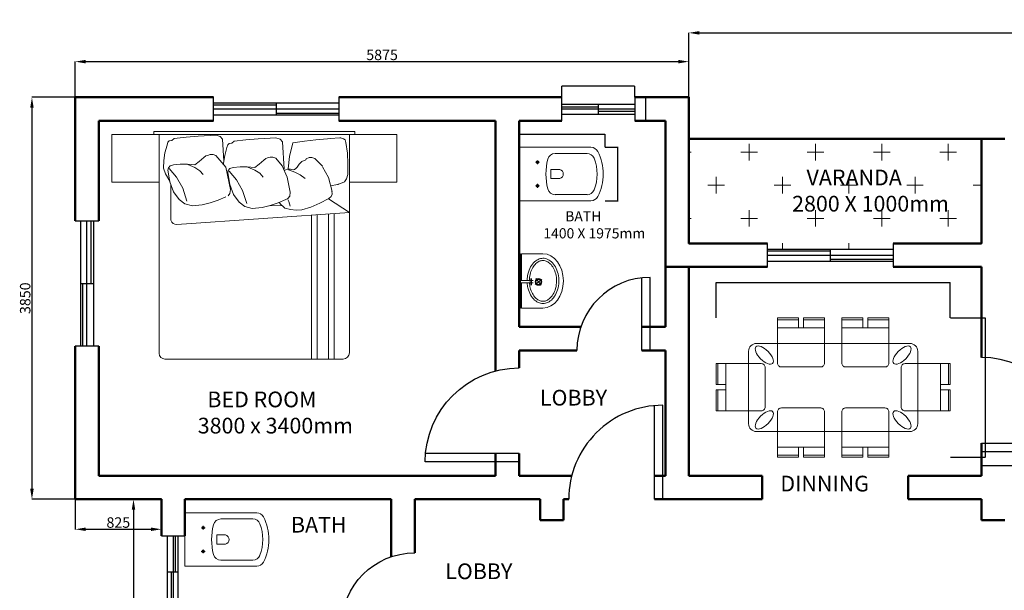
# Model space of a CAD drawing. Units: millimetres. Extents: x -857 to 54106, y -13666 to 13947.
# Tile 11 of 41: x 2211 to 11637, y 8482 to 13947. Entities that reach past the tile are written whole.
import ezdxf

# ---------------------------------------------------------------- set-up
doc = ezdxf.new("R2010")
doc.units = ezdxf.units.MM
for name, color, linetype, lineweight in [('A-ANNO-DIMS', 2, 'Continuous', 18), ('A-AREA-IDEN', 3, 'Continuous', 18), ('A-DOOR', 1, 'Continuous', 25), ('A-FLOR-FIXT', 8, 'Continuous', 18), ('A-FLOR-PATT', 252, 'Continuous', 13), ('A-FURN', 21, 'Continuous', 18), ('A-FURNITURE', 25, 'Continuous', 9), ('A-GLAZ', 4, 'Continuous', 25), ('A-SANITARY FITTINGS', 25, 'Continuous', 15), ('A-WALL', 7, 'Continuous', 50)]:
    doc.layers.add(name, color=color, linetype=linetype, lineweight=lineweight)
doc.styles.get("Standard").update_dxf_attribs({"font": 'arial.ttf'})
doc.dimstyles.new('ISO-25', dxfattribs={"dimtxt": 2.5, "dimasz": 2.5, "dimexe": 1.25, "dimexo": 0.625, "dimtad": 1, "dimtxsty": 'Standard', "dimcen": 2.5, "dimadec": 0, "dimazin": 0, "dimtfac": 1, "dimtmove": 0, "dimatfit": 3, "dimfxl": 1, "dimarcsym": 0})

# ---------------------------------------------------------------- blocks, each defined once
blk = doc.blocks.new('dasd')
at = {"layer": 'A-FURNITURE'}
for p, q in [((-12.51, 13.31), (-12.51, 2.88)), ((-3.95, 13.31), (-12.51, 13.31)), ((-3.95, 12.51), (-12.51, 12.51)), ((-3.95, 9.3), (-3.95, 13.31)), ((6.74, 13.31), (-1.81, 13.31)), ((-1.81, 9.3), (-1.81, 13.31)), ((6.74, 12.51), (-1.81, 12.51)), ((6.74, 2.88), (6.74, 13.31)), ((6.74, 9.3), (-12.51, 9.3)), ((-21, -11.75), (-31.43, -11.75)), ((-31.43, -11.75), (-31.43, -20.3)), ((-30.63, -11.75), (-30.63, -20.3)), ((-27.42, -11.75), (-27.42, -31)), ((15, -11.75), (25.43, -11.75)), ((21.42, -11.75), (21.42, -31)), ((24.63, -11.75), (24.63, -20.3)), ((25.43, -11.75), (25.43, -20.3)), ((-27.42, -20.3), (-31.43, -20.3)), ((-31.43, -22.44), (-31.43, -31)), ((-27.42, -22.44), (-31.43, -22.44)), ((-30.63, -22.44), (-30.63, -31)), ((21.42, -20.3), (25.43, -20.3)), ((21.42, -22.44), (25.43, -22.44)), ((24.63, -22.44), (24.63, -31)), ((25.43, -22.44), (25.43, -31)), ((-31.43, -31), (-21, -31)), ((25.43, -31), (15, -31)), ((-21, -38), (-31.43, -38)), ((-31.43, -38), (-31.43, -46.55)), ((-30.63, -38), (-30.63, -46.55)), ((-27.42, -38), (-27.42, -57.25)), ((15, -38), (25.43, -38)), ((21.42, -38), (21.42, -57.25)), ((24.63, -38), (24.63, -46.55)), ((25.43, -38), (25.43, -46.55)), ((-27.42, -46.55), (-31.43, -46.55)), ((21.42, -46.55), (25.43, -46.55)), ((-31.43, -48.69), (-31.43, -57.25)), ((-27.42, -48.69), (-31.43, -48.69)), ((-30.63, -48.69), (-30.63, -57.25)), ((21.42, -48.69), (25.43, -48.69)), ((24.63, -48.69), (24.63, -57.25)), ((25.43, -48.69), (25.43, -57.25)), ((-31.43, -57.25), (-21, -57.25)), ((25.43, -57.25), (15, -57.25)), ((-12.51, -82.31), (-12.51, -71.88)), ((6.74, -71.88), (6.74, -82.31)), ((6.74, -78.3), (-12.51, -78.3)), ((-3.95, -78.3), (-3.95, -82.31)), ((-1.81, -78.3), (-1.81, -82.31)), ((-3.95, -81.51), (-12.51, -81.51)), ((-3.95, -82.31), (-12.51, -82.31)), ((6.74, -81.51), (-1.81, -81.51)), ((6.74, -82.31), (-1.81, -82.31))]:
    blk.add_line(p, q, dxfattribs=at)
blk.add_lwpolyline([(-21, -65.79), (-21, -3.21, -0.414214), (-17.79, 0), (11.79, 0, -0.414214), (15, -3.21), (15, -65.79, -0.414214), (11.79, -69), (-17.79, -69, -0.414214)], format="xyb", close=True, dxfattribs=at)
at = {"layer": 'A-FURNITURE', "ltscale": 5}
for points in [[(-12.51, 2.88), (-12.51, -5.14, 0.414214), (-10.91, -6.74), (5.14, -6.74, 0.414214), (6.74, -5.14), (6.74, 2.88)], [(-21, -31), (-12.98, -31, 0.414214), (-11.37, -29.4), (-11.37, -13.35, 0.414214), (-12.98, -11.75), (-21, -11.75)], [(15, -31), (6.98, -31, -0.414214), (5.37, -29.4), (5.37, -13.35, -0.414214), (6.98, -11.75), (15, -11.75)], [(-21, -57.25), (-12.98, -57.25, 0.414214), (-11.37, -55.65), (-11.37, -39.6, 0.414214), (-12.98, -38), (-21, -38)], [(15, -57.25), (6.98, -57.25, -0.414214), (5.37, -55.65), (5.37, -39.6, -0.414214), (6.98, -38), (15, -38)], [(-12.51, -71.88), (-12.51, -63.86, -0.414214), (-10.91, -62.26), (5.14, -62.26, -0.414214), (6.74, -63.86), (6.74, -71.88)]]:
    blk.add_lwpolyline(points, format="xyb", dxfattribs=at)
for centre, major_axis in [((-16.23, -6.4), (-3.4, 3.4)), ((10.23, -62.6), (3.4, -3.4))]:
    blk.add_ellipse(centre, major_axis=major_axis, ratio=0.444444, dxfattribs=at)
at = {"layer": 'A-FURNITURE', "ltscale": 5, "extrusion": (0, 0, -1)}
for centre, major_axis in [((10.23, -6.4), (3.4, 3.4)), ((-16.23, -62.6), (-3.4, -3.4))]:
    blk.add_ellipse(centre, major_axis=major_axis, ratio=0.444444, dxfattribs=at)
blk = doc.blocks.new('A$C7d9d00ca')
at = {"layer": 'A-SANITARY FITTINGS'}
for p, q in [((0, 0), (-13.78, 0)), ((-13.78, -18.49), (-13.78, 0)), ((0, -18.49), (0, 0)), ((-10.42, -4.72), (-9.43, -4.72)), ((-9.94, -4.23), (-9.94, -5.23)), ((-3.36, -4.73), (-4.34, -4.73)), ((-3.84, -4.24), (-3.84, -5.24)), ((-12.2, -9.27), (-12.2, -17.48)), ((-1.57, -9.27), (-1.57, -17.48))]:
    blk.add_line(p, q, dxfattribs=at)
for points in [[(-8.08, -8.19), (-5.7, -8.19), (-5.7, -8.19), (-5.7, -10.48)], [(-8.08, -8.19), (-8.08, -10.48)]]:
    blk.add_lwpolyline(points, dxfattribs=at)
for centre in [(-9.94, -4.72), (-3.84, -4.73)]:
    blk.add_circle(centre, 0.342, dxfattribs=at)
for centre, radius, start, end in [((-10.24, -9.27), 1.97, 103.8652, 180), ((-6.89, -22.82), 15.93, 76.135, 103.8652), ((-3.54, -9.27), 1.97, 0.0003, 76.135), ((-6.89, -10.13), 1.24, 196.5098, 343.4902), ((-10.24, -17.48), 1.97, 180, 248.6555), ((-3.54, -17.48), 1.97, 291.3447, 0.0003), ((-11.81, -18.49), 1.97, 180, 242.8074), ((-6.89, -8.92), 12.74, 242.8074, 297.1926), ((-6.89, -8.92), 11.16, 248.6555, 291.3447), ((-1.97, -18.49), 1.97, 297.1926, 0)]:
    blk.add_arc(centre, radius, start, end, dxfattribs=at)
blk = doc.blocks.new('A$C0124305E')
at = {"layer": 'A-SANITARY FITTINGS'}
for p, q in [((-8.42, 16.01), (-0.8, 16.01)), ((-0.8, 7.08), (-0.8, 16.01)), ((-5.66, 7.68), (-8, 5.88)), ((-7.73, 7.95), (-5.93, 5.62)), ((0, 7.08), (-4.99, 7.08)), ((-4.31, 5.61), (-4.31, 7.96)), ((-3.91, 5.61), (-3.91, 7.96)), ((0, 6.28), (-4.99, 6.28)), ((-0.8, -3.19), (-0.8, 6.28)), ((-8.42, -3.19), (-0.8, -3.19))]:
    blk.add_line(p, q, dxfattribs=at)
blk.add_lwpolyline([(-0.5, 16.01), (0, 16.01), (0, -3.19), (-0.5, -3.19)], close=True, dxfattribs=at)
for radius in [1.18, 0.885]:
    blk.add_circle((-6.83, 6.78), radius, dxfattribs=at)
at = {"layer": 'A-SANITARY FITTINGS', "extrusion": (0, 0, -1)}
blk.add_ellipse((-8.42, 6.41), major_axis=(0, 9.6), ratio=0.75, start_param=3.141593, end_param=6.283185, dxfattribs=at)
at = {"layer": 'A-SANITARY FITTINGS'}
for points, knots in [([(-2.82, 6.28), (-2.82, 5.74), (-2.87, 5.2), (-3.1, 3.74), (-3.37, 2.86), (-4.09, 1.28), (-4.55, 0.6), (-5.56, -0.5), (-6.12, -0.92), (-7.25, -1.45), (-7.83, -1.58), (-8.98, -1.59), (-9.55, -1.46), (-10.69, -0.93), (-11.25, -0.52), (-12.27, 0.57), (-12.72, 1.25), (-13.45, 2.82), (-13.72, 3.71), (-14.02, 5.56), (-14.05, 6.52), (-13.88, 8.41), (-13.67, 9.32), (-13.04, 10.99), (-12.62, 11.73), (-11.66, 12.96), (-11.12, 13.45), (-10, 14.13), (-9.43, 14.32), (-8.28, 14.45), (-7.7, 14.39), (-6.56, 14), (-5.99, 13.66), (-4.93, 12.71), (-4.44, 12.09), (-3.62, 10.62), (-3.3, 9.78), (-2.96, 8.29), (-2.87, 7.69), (-2.84, 7.08)], [1.58652, 1.58652, 1.58652, 1.58652, 1.780321, 1.780321, 2.120053, 2.120053, 2.459785, 2.459785, 2.799517, 2.799517, 3.139249, 3.139249, 3.478981, 3.478981, 3.818713, 3.818713, 4.158445, 4.158445, 4.498177, 4.498177, 4.837909, 4.837909, 5.177641, 5.177641, 5.517373, 5.517373, 5.857105, 5.857105, 6.196837, 6.196837, 6.536569, 6.536569, 6.876301, 6.876301, 7.216033, 7.216033, 7.555765, 7.555765, 7.774364, 7.774364, 7.774364, 7.774364]), ([(-3.62, 6.29), (-3.62, 5.76), (-3.67, 5.23), (-3.88, 3.96), (-4.1, 3.23), (-4.65, 1.95), (-4.98, 1.39), (-5.72, 0.46), (-6.12, 0.1), (-6.92, -0.44), (-7.32, -0.61), (-8.11, -0.8), (-8.5, -0.81), (-9.28, -0.69), (-9.68, -0.55), (-10.48, -0.08), (-10.89, 0.24), (-11.67, 1.13), (-12.05, 1.7), (-12.66, 3.01), (-12.9, 3.76), (-13.2, 5.38), (-13.25, 6.28), (-13.13, 8.02), (-12.95, 8.88), (-12.42, 10.42), (-12.06, 11.12), (-11.23, 12.25), (-10.77, 12.7), (-9.92, 13.26), (-9.53, 13.43), (-8.78, 13.62), (-8.41, 13.64), (-7.66, 13.54), (-7.28, 13.42), (-6.51, 13.02), (-6.12, 12.73), (-5.35, 11.95), (-4.97, 11.43), (-4.34, 10.23), (-4.08, 9.54), (-3.76, 8.24), (-3.67, 7.64), (-3.63, 7.03)], [1.58652, 1.58652, 1.58652, 1.58652, 1.790653, 1.790653, 2.093007, 2.093007, 2.384527, 2.384527, 2.676047, 2.676047, 2.967567, 2.967567, 3.259087, 3.259087, 3.550608, 3.550608, 3.842128, 3.842128, 4.155456, 4.155456, 4.468784, 4.468784, 4.806699, 4.806699, 5.144614, 5.144614, 5.482529, 5.482529, 5.820444, 5.820444, 6.099515, 6.099515, 6.378586, 6.378586, 6.657656, 6.657656, 6.936727, 6.936727, 7.23864, 7.23864, 7.540552, 7.540552, 7.774364, 7.774364, 7.774364, 7.774364])]:
    blk.add_open_spline(points, degree=3, knots=knots, dxfattribs=at)
blk = doc.blocks.new('A$C06e6df2d')
at = {"layer": 'A-FURNITURE'}
for p, q in [((-75.01, 24.58), (-75.01, 68.89)), ((-73.01, 70.89), (-16.87, 70.89)), ((-70.22, 24.92), (-70.22, 70.89)), ((-68.43, 25.04), (-68.43, 70.89)), ((-64.83, 25.3), (-64.83, 70.89)), ((-63.04, 25.42), (-63.04, 70.89)), ((-15.01, 0), (-15.01, 69.09)), ((-75.01, 24.58), (-20.56, 28.42)), ((-18.69, 15.78), (-18.71, 27.06)), ((-68.39, 20.29), (-75.01, 24.58)), ((-75.01, 24.58), (-75.01, 0)), ((-65.73, 21.73), (-62.87, 22.91)), ((-62.87, 22.91), (-59.95, 23.77)), ((-59.95, 23.77), (-58.19, 23.92)), ((-58.19, 23.92), (-56.43, 23.73)), ((-56.43, 23.73), (-54.68, 23.22)), ((-56.16, 21.87), (-56.3, 22.64)), ((-55.9, 21.17), (-56.16, 21.87)), ((-54.68, 23.22), (-54.09, 22.72)), ((-54.09, 22.72), (-53.51, 22.17)), ((-49.77, 22.5), (-53.75, 22.43)), ((-53.51, 22.17), (-52.8, 21.44)), ((-52.5, 21.58), (-50.02, 22.42)), ((-50.02, 22.42), (-47.49, 23.05)), ((-47.49, 23.05), (-44.37, 23.33)), ((-44.37, 23.33), (-41.97, 22.72)), ((-41.32, 17.73), (-42.66, 21.83)), ((-41.97, 22.72), (-40.19, 21.34)), ((-31.12, 21.59), (-28.59, 22.22)), ((-28.59, 22.22), (-25.48, 22.5)), ((-25.48, 22.5), (-23.07, 21.9)), ((-23.07, 21.9), (-21.29, 20.51)), ((-69.62, 18.81), (-69.3, 19.62)), ((-69.5, 17.78), (-69.62, 18.81)), ((-69.3, 19.62), (-68.53, 20.21)), ((-68.53, 20.21), (-65.73, 21.73)), ((-56.34, 18.24), (-56.19, 19.49)), ((-56.19, 19.49), (-55.62, 20.16)), ((-55.54, 20.51), (-55.9, 21.17)), ((-55.62, 20.16), (-54.92, 20.5)), ((-54.92, 20.5), (-52.5, 21.58)), ((-40.19, 21.34), (-38.45, 18.93)), ((-38.45, 18.93), (-37.3, 15.81)), ((-37.44, 17.41), (-37.29, 18.66)), ((-37.29, 18.66), (-36.72, 19.34)), ((-36.02, 19.68), (-33.6, 20.75)), ((-33.6, 20.75), (-31.12, 21.59)), ((-22.42, 16.9), (-23.76, 21)), ((-21.29, 20.51), (-19.55, 18.1)), ((-71.64, 15.67), (-73.5, 14.91)), ((-71.25, 15.78), (-71.44, 15.74)), ((-69.05, 16.16), (-71.23, 15.78)), ((-68.39, 13.59), (-69.52, 17.98)), ((-55.37, 13.49), (-56.34, 18.24)), ((-39.4, 14.32), (-41.32, 17.73)), ((-35.98, 10.29), (-37.44, 17.41)), ((-37.3, 15.81), (-36.66, 12.07)), ((-20.5, 13.49), (-22.42, 16.9)), ((-19.55, 18.1), (-18.4, 14.98)), ((-74.47, 12.68), (-74.56, 9.28)), ((-74.12, 14.04), (-74.47, 12.68)), ((-73.5, 14.91), (-74.12, 14.04)), ((-66.57, 10.23), (-68.39, 13.59)), ((-61.02, 13.94), (-59.51, 12.79)), ((-59.51, 12.79), (-57.79, 11.86)), ((-53.83, 9.92), (-55.37, 13.49)), ((-47.81, 13.43), (-46.76, 12.26)), ((-37.06, 11.55), (-39.4, 14.32)), ((-28.91, 12.6), (-27.86, 11.44)), ((-18.16, 10.72), (-20.5, 13.49)), ((-18.4, 14.98), (-17.76, 11.24)), ((-16.95, 12.45), (-18.35, 14.73)), ((-16.34, 10.65), (-16.95, 12.45)), ((-64.09, 7.63), (-66.55, 10.02)), ((-59.16, 9.35), (-60.04, 8.55)), ((-58.52, 10.37), (-59.16, 9.35)), ((-58.11, 10.75), (-58.52, 10.37)), ((-57.7, 11.01), (-58.11, 10.75)), ((-57.79, 11.86), (-55.84, 11.15)), ((-57.28, 11.14), (-57.7, 11.01)), ((-56.4, 10.96), (-57.28, 11.14)), ((-55.52, 11), (-56.4, 10.96)), ((-56.14, 6.96), (-55.7, 10.85)), ((-54.44, 11.32), (-55.52, 11)), ((-54.44, 10.96), (-53.85, 2.28)), ((-51.75, 7.51), (-53.83, 9.92)), ((-46.52, 9.32), (-47.98, 8.12)), ((-46.76, 12.26), (-45.12, 11.25)), ((-45.15, 10.44), (-46.52, 9.32)), ((-42.78, 10.21), (-45.15, 10.44)), ((-45.12, 11.25), (-42.96, 10.31)), ((-40.52, 10.2), (-42.78, 10.21)), ((-38.37, 10.42), (-40.52, 10.2)), ((-37.33, 10.73), (-38.37, 10.42)), ((-36.79, 11.34), (-37.33, 10.73)), ((-36.66, 12.07), (-36.79, 11.34)), ((-32.85, 6.68), (-35.98, 10.29)), ((-35.33, 9.04), (-35.31, 9.52)), ((-27.86, 11.44), (-26.22, 10.43)), ((-26.26, 9.61), (-27.62, 8.5)), ((-23.88, 9.38), (-26.26, 9.61)), ((-26.22, 10.43), (-24.06, 9.48)), ((-21.62, 9.38), (-23.88, 9.38)), ((-19.47, 9.59), (-21.62, 9.38)), ((-18.43, 9.9), (-19.47, 9.59)), ((-17.89, 10.51), (-18.43, 9.9)), ((-17.76, 11.24), (-17.89, 10.51)), ((-16.43, 8.21), (-16.34, 10.65)), ((-74.56, 9.28), (-74.36, 5.88)), ((-63.18, 7.26), (-64.09, 7.63)), ((-62.27, 7.28), (-63.18, 7.26)), ((-61.35, 7.68), (-62.27, 7.28)), ((-61.24, 7.96), (-61.35, 7.68)), ((-60.04, 8.55), (-61.24, 7.96)), ((-57.17, 2.61), (-56.14, 6.96)), ((-50.88, 7.2), (-51.75, 7.51)), ((-50.02, 7.17), (-50.88, 7.2)), ((-49.15, 7.42), (-50.02, 7.17)), ((-48.66, 7.55), (-49.15, 7.42)), ((-47.98, 8.12), (-48.66, 7.55)), ((-36.37, 4.16), (-35.72, 6.6)), ((-35.72, 6.6), (-35.33, 9.04)), ((-35.43, 8.42), (-34.95, 1.45)), ((-31.98, 6.37), (-32.85, 6.68)), ((-31.12, 6.34), (-31.98, 6.37)), ((-30.25, 6.59), (-31.12, 6.34)), ((-29.76, 6.73), (-30.25, 6.59)), ((-29.08, 7.29), (-29.76, 6.73)), ((-27.62, 8.5), (-29.08, 7.29)), ((-16.82, 5.77), (-16.43, 8.21)), ((-74.36, 5.88), (-73.9, 2.49)), ((-37.09, 2.83), (-36.6, 3.27)), ((-36.6, 3.27), (-36.37, 4.16)), ((-17.71, 2.44), (-17.47, 3.33)), ((-17.47, 3.33), (-16.82, 5.77)), ((-76.74, 0), (-76.74, -0.9)), ((-13.27, 0), (-76.74, 0)), ((-73.9, 2.49), (-73.65, 1.74)), ((-73.65, 1.74), (-73.12, 1.41)), ((-71.96, 1.11), (-68.94, 1.26)), ((-68.94, 1.26), (-68.06, 1.33)), ((-68.06, 1.33), (-64.46, 1.68)), ((-64.46, 1.68), (-60.83, 2.11)), ((-60.83, 2.11), (-57.17, 2.61)), ((-53.85, 2.28), (-53.12, 1.45)), ((-53.12, 1.45), (-51.84, 1.07)), ((-51.84, 1.07), (-49.99, 1.14)), ((-49.99, 1.14), (-46.17, 1.35)), ((-46.17, 1.35), (-42.37, 1.69)), ((-42.37, 1.69), (-38.61, 2.15)), ((-38.61, 2.15), (-37.87, 2.73)), ((-37.87, 2.73), (-37.09, 2.83)), ((-34.95, 1.45), (-34.22, 0.63)), ((-34.22, 0.63), (-32.94, 0.25)), ((-32.94, 0.25), (-31.09, 0.31)), ((-31.09, 0.31), (-27.27, 0.52)), ((-27.27, 0.52), (-23.47, 0.86)), ((-23.47, 0.86), (-19.71, 1.32)), ((-19.71, 1.32), (-18.97, 1.91)), ((-18.97, 1.91), (-18.19, 2.01)), ((-18.19, 2.01), (-17.71, 2.44)), ((-13.27, -0.9), (-13.27, 0)), ((-13.27, -0.9), (-76.74, -0.9))]:
    blk.add_line(p, q, dxfattribs=at)
for points in [[(-75.01, 0), (-90.01, 0), (-90.01, 15.01), (-75.01, 15.01)], [(-15.01, 0), (0, 0), (0, 15.01), (-15.01, 15.01)]]:
    blk.add_lwpolyline(points, close=True, dxfattribs=at)
for centre, radius, start, end in [((-73.01, 68.89), 2, 90, 180), ((-16.8, 69.09), 1.8, 0, 90), ((-20.45, 26.63), 1.8, 13.7792, 93.47), ((-70.89, 13.81), 2, 99.8546, 112.1195), ((-72.06, 3.1), 2, 238.0354, 272.9353)]:
    blk.add_arc(centre, radius, start, end, dxfattribs=at)
blk = doc.blocks.new('*D20')
at = {"layer": 'A-ANNO-DIMS', "color": 0, "lineweight": -2, "transparency": 16777216}
for p, q in [((2742.3, 13204.9), (2742.3, 13546.1)), ((2842.3, 13544.9), (8517.3, 13544.9)), ((8617.3, 13204.9), (8617.3, 13546.1))]:
    blk.add_line(p, q, dxfattribs=at)
at = {"layer": 'A-ANNO-DIMS', "color": 0, "transparency": 16777216}
for points in [[(2842.3, 13561.5), (2842.3, 13528.2), (2742.3, 13544.9)], [(8517.3, 13561.5), (8517.3, 13528.2), (8617.3, 13544.9)]]:
    blk.add_solid(points, dxfattribs=at)
at = {"layer": 'Defpoints', "color": 0, "transparency": 16777216}
for p in [(8617.3, 13544.9), (2742.3, 13204.2), (8617.3, 13204.2)]:
    blk.add_point(p, dxfattribs=at)
at = {"layer": 'A-ANNO-DIMS', "color": 0, "transparency": 16777216, "insert": (5679.8, 13596.5), "char_height": 100, "attachment_point": 5}
blk.add_mtext('5875', dxfattribs=at)
blk = doc.blocks.new('*D21')
at = {"layer": 'A-ANNO-DIMS', "color": 0, "lineweight": -2, "transparency": 16777216}
for p, q in [((2741.7, 13204.2), (2326.7, 13204.2)), ((2328, 13104.2), (2328, 9454.2)), ((2741.7, 9354.2), (2326.7, 9354.2))]:
    blk.add_line(p, q, dxfattribs=at)
at = {"layer": 'A-ANNO-DIMS', "color": 0, "transparency": 16777216}
for points in [[(2311.3, 13104.2), (2344.6, 13104.2), (2328, 13204.2)], [(2311.3, 9454.2), (2344.6, 9454.2), (2328, 9354.2)]]:
    blk.add_solid(points, dxfattribs=at)
at = {"layer": 'Defpoints', "color": 0, "transparency": 16777216}
for p in [(2742.3, 13204.2), (2328, 9354.2), (2742.3, 9354.2)]:
    blk.add_point(p, dxfattribs=at)
at = {"layer": 'A-ANNO-DIMS', "color": 0, "transparency": 16777216, "insert": (2276.2, 11279.2), "char_height": 100, "attachment_point": 5, "rotation": 90}
blk.add_mtext('3850', dxfattribs=at)
blk = doc.blocks.new('*D22')
at = {"layer": 'A-ANNO-DIMS', "color": 0, "lineweight": -2, "transparency": 16777216}
for p, q in [((2742.3, 9353.6), (2742.3, 9065.3)), ((3567.3, 9353.6), (3567.3, 9065.3)), ((2842.3, 9066.5), (3467.3, 9066.5))]:
    blk.add_line(p, q, dxfattribs=at)
at = {"layer": 'A-ANNO-DIMS', "color": 0, "transparency": 16777216}
for points in [[(2842.3, 9083.2), (2842.3, 9049.8), (2742.3, 9066.5)], [(3467.3, 9083.2), (3467.3, 9049.8), (3567.3, 9066.5)]]:
    blk.add_solid(points, dxfattribs=at)
at = {"layer": 'Defpoints', "color": 0, "transparency": 16777216}
for p in [(2742.3, 9354.2), (3567.3, 9354.2), (3567.3, 9066.5)]:
    blk.add_point(p, dxfattribs=at)
at = {"layer": 'A-ANNO-DIMS', "color": 0, "transparency": 16777216, "insert": (3154.8, 9118.2), "char_height": 100, "attachment_point": 5}
blk.add_mtext('825', dxfattribs=at)
blk = doc.blocks.new('*D23')
at = {"layer": 'A-ANNO-DIMS', "color": 0, "lineweight": -2, "transparency": 16777216}
for p, q in [((3566.7, 9354.2), (3298.9, 9354.2)), ((3300.1, 9254.2), (3300.1, 4004.3)), ((3566, 3904.3), (3298.9, 3904.3))]:
    blk.add_line(p, q, dxfattribs=at)
at = {"layer": 'A-ANNO-DIMS', "color": 0, "transparency": 16777216}
for points in [[(3283.5, 9254.2), (3316.8, 9254.2), (3300.1, 9354.2)], [(3283.5, 4004.3), (3316.8, 4004.3), (3300.1, 3904.3)]]:
    blk.add_solid(points, dxfattribs=at)
at = {"layer": 'Defpoints', "color": 0, "transparency": 16777216}
for p in [(3567.3, 9354.2), (3300.1, 3904.3), (3566.6, 3904.3)]:
    blk.add_point(p, dxfattribs=at)
at = {"layer": 'A-ANNO-DIMS', "color": 0, "transparency": 16777216, "insert": (3239.4, 6629.2), "char_height": 100, "attachment_point": 5, "rotation": 90}
blk.add_mtext('5449,97', dxfattribs=at)
blk = doc.blocks.new('*D25')
at = {"layer": 'A-ANNO-DIMS', "color": 0, "lineweight": -2, "transparency": 16777216}
for p, q in [((8617.3, 12804.9), (8617.3, 13821.5)), ((8717.3, 13820.3), (16292.3, 13820.3)), ((16392.3, 12804.9), (16392.3, 13821.5))]:
    blk.add_line(p, q, dxfattribs=at)
at = {"layer": 'A-ANNO-DIMS', "color": 0, "transparency": 16777216}
for points in [[(8717.3, 13837), (8717.3, 13803.6), (8617.3, 13820.3)], [(16292.3, 13837), (16292.3, 13803.6), (16392.3, 13820.3)]]:
    blk.add_solid(points, dxfattribs=at)
at = {"layer": 'Defpoints', "color": 0, "transparency": 16777216}
for p in [(16392.3, 13820.3), (8617.3, 12804.2), (16392.3, 12804.2)]:
    blk.add_point(p, dxfattribs=at)
at = {"layer": 'A-ANNO-DIMS', "color": 0, "transparency": 16777216, "insert": (12504.8, 13881), "char_height": 100, "attachment_point": 5}
blk.add_mtext('7774,98', dxfattribs=at)
blk = doc.blocks.new('DOOR-900')
blk.add_line((11417.3, 9811.5), (12317.3, 9811.5))
blk.add_arc((11417.3, 9811.5), 900, 0, 90)
blk = doc.blocks.new('DOOR-700')
blk.add_line((8245.5, 10779.2), (8245.5, 11479.2))
blk.add_arc((8245.5, 10779.2), 700, 90, 180)
blk = doc.blocks.new('WIN-1200')
for p, q in [((9371.3, 11750.2), (10571.3, 11750.2)), ((9371.3, 11731.7), (9971.3, 11731.7)), ((9371.3, 11691.7), (10571.3, 11691.7)), ((9971.3, 11750.2), (9971.3, 11630.7)), ((10571.3, 11630.7), (9371.3, 11630.7)), ((9971.3, 11651.7), (10571.3, 11651.7))]:
    blk.add_line(p, q)
for points in [[(9371.3, 11579.2), (9371.3, 11804.2)], [(10571.3, 11804.2), (10571.3, 11579.2)]]:
    blk.add_lwpolyline(points)
blk = doc.blocks.new('WIN-700')
for p, q in [((3626.3, 8304.2), (3626.3, 9004.2)), ((3679.8, 9004.2), (3679.8, 8304.2)), ((3699.8, 9004.2), (3699.8, 8654.2)), ((3724.4, 9004.2), (3724.4, 8304.2)), ((3724.4, 8654.2), (3626.3, 8654.2)), ((3659.8, 8654.2), (3659.8, 8304.2))]:
    blk.add_line(p, q)
for points in [[(3567.3, 9004.2), (3792.3, 9004.2)], [(3792.3, 8304.2), (3567.3, 8304.2)]]:
    blk.add_lwpolyline(points)
blk = doc.blocks.new('*D31')
at = {"layer": 'A-ANNO-DIMS', "color": 0, "lineweight": -2, "transparency": 16777216}
for p, q in [((11417.3, 9810.9), (11417.3, 9675.2)), ((12317.3, 9810.9), (12317.3, 9675.2)), ((11419.8, 9676.5), (12314.8, 9676.5))]:
    blk.add_line(p, q, dxfattribs=at)
at = {"layer": 'A-ANNO-DIMS', "color": 0, "transparency": 16777216}
for points in [[(11419.8, 9676.9), (11419.8, 9676.1), (11417.3, 9676.5)], [(12314.8, 9676.9), (12314.8, 9676.1), (12317.3, 9676.5)]]:
    blk.add_solid(points, dxfattribs=at)
at = {"layer": 'Defpoints', "color": 0, "transparency": 16777216}
for p in [(11417.3, 9811.5), (12317.3, 9811.5), (12317.3, 9676.5)]:
    blk.add_point(p, dxfattribs=at)
at = {"layer": 'A-ANNO-DIMS', "color": 0, "transparency": 16777216, "insert": (11867.3, 9678.4), "char_height": 2.5, "attachment_point": 5}
blk.add_mtext('DOOR D1 900 TYP.', dxfattribs=at)
blk = doc.blocks.new('*D37')
at = {"layer": 'A-ANNO-DIMS', "color": 0, "lineweight": -2, "transparency": 16777216}
for p, q in [((7399.4, 13204.9), (7399.4, 13310.5)), ((8096.9, 13309.2), (7401.9, 13309.2)), ((8099.4, 13204.9), (8099.4, 13310.5))]:
    blk.add_line(p, q, dxfattribs=at)
at = {"layer": 'A-ANNO-DIMS', "color": 0, "transparency": 16777216}
for points in [[(7401.9, 13309.6), (7401.9, 13308.8), (7399.4, 13309.2)], [(8096.9, 13309.6), (8096.9, 13308.8), (8099.4, 13309.2)]]:
    blk.add_solid(points, dxfattribs=at)
at = {"layer": 'Defpoints', "color": 0, "transparency": 16777216}
for p in [(7399.4, 13309.2), (7399.4, 13204.2), (8099.4, 13204.2)]:
    blk.add_point(p, dxfattribs=at)
at = {"layer": 'A-ANNO-DIMS', "color": 0, "transparency": 16777216, "insert": (7749.4, 13311.1), "char_height": 2.5, "attachment_point": 5}
blk.add_mtext('WINDOW W2 700 TYP.', dxfattribs=at)
blk = doc.blocks.new('*D38')
at = {"layer": 'A-ANNO-DIMS', "color": 0, "lineweight": -2, "transparency": 16777216}
for p, q in [((8100.1, 13204.2), (8205.7, 13204.2)), ((8204.4, 12981.7), (8204.4, 13201.7)), ((8100.1, 12979.2), (8205.7, 12979.2))]:
    blk.add_line(p, q, dxfattribs=at)
at = {"layer": 'A-ANNO-DIMS', "color": 0, "transparency": 16777216}
for points in [[(8204, 13201.7), (8204.9, 13201.7), (8204.4, 13204.2)], [(8204, 12981.7), (8204.9, 12981.7), (8204.4, 12979.2)]]:
    blk.add_solid(points, dxfattribs=at)
at = {"layer": 'Defpoints', "color": 0, "transparency": 16777216}
for p in [(8099.4, 13204.2), (8204.4, 13204.2), (8099.4, 12979.2)]:
    blk.add_point(p, dxfattribs=at)
at = {"layer": 'A-ANNO-DIMS', "color": 0, "transparency": 16777216, "insert": (8202.5, 13091.7), "char_height": 2.5, "attachment_point": 5, "rotation": 90}
blk.add_mtext('225 TYP.', dxfattribs=at)
blk = doc.blocks.new('*D39')
at = {"layer": 'A-ANNO-DIMS', "color": 0, "lineweight": -2, "transparency": 16777216}
for p, q in [((6992.3, 12725), (6992.3, 12849)), ((7811.8, 12847.7), (6994.8, 12847.7)), ((7814.3, 12725), (7814.3, 12849))]:
    blk.add_line(p, q, dxfattribs=at)
at = {"layer": 'A-ANNO-DIMS', "color": 0, "transparency": 16777216}
for points in [[(6994.8, 12848.1), (6994.8, 12847.3), (6992.3, 12847.7)], [(7811.8, 12848.1), (7811.8, 12847.3), (7814.3, 12847.7)]]:
    blk.add_solid(points, dxfattribs=at)
at = {"layer": 'Defpoints', "color": 0, "transparency": 16777216}
for p in [(6992.3, 12847.7), (6992.3, 12724.4), (7814.3, 12724.4)]:
    blk.add_point(p, dxfattribs=at)
at = {"layer": 'A-ANNO-DIMS', "color": 0, "transparency": 16777216, "insert": (7403.3, 12849.6), "char_height": 2.5, "attachment_point": 5}
blk.add_mtext('WC 822 TYP.', dxfattribs=at)
blk = doc.blocks.new('*D40')
at = {"layer": 'A-ANNO-DIMS', "color": 0, "lineweight": -2, "transparency": 16777216}
for p, q in [((7814.9, 12724.4), (7938.9, 12724.4)), ((7937.6, 12214.9), (7937.6, 12721.9)), ((7814.9, 12212.4), (7938.9, 12212.4))]:
    blk.add_line(p, q, dxfattribs=at)
at = {"layer": 'A-ANNO-DIMS', "color": 0, "transparency": 16777216}
for points in [[(7937.2, 12721.9), (7938, 12721.9), (7937.6, 12724.4)], [(7937.2, 12214.9), (7938, 12214.9), (7937.6, 12212.4)]]:
    blk.add_solid(points, dxfattribs=at)
at = {"layer": 'Defpoints', "color": 0, "transparency": 16777216}
for p in [(7814.3, 12724.4), (7937.6, 12724.4), (7814.3, 12212.4)]:
    blk.add_point(p, dxfattribs=at)
at = {"layer": 'A-ANNO-DIMS', "color": 0, "transparency": 16777216, "insert": (7935.7, 12468.4), "char_height": 2.5, "attachment_point": 5, "rotation": 90}
blk.add_mtext('512 TYP.', dxfattribs=at)
blk = doc.blocks.new('*D51')
at = {"layer": 'A-ANNO-DIMS', "color": 0, "lineweight": -2, "transparency": 16777216}
for p, q in [((8877, 11091.7), (8877, 11428.8)), ((11117.3, 11427.5), (8879.5, 11427.5)), ((11119.8, 11091.7), (11119.8, 11428.8))]:
    blk.add_line(p, q, dxfattribs=at)
at = {"layer": 'A-ANNO-DIMS', "color": 0, "transparency": 16777216}
for points in [[(8879.5, 11427.9), (8879.5, 11427.1), (8877, 11427.5)], [(11117.3, 11427.9), (11117.3, 11427.1), (11119.8, 11427.5)]]:
    blk.add_solid(points, dxfattribs=at)
at = {"layer": 'Defpoints', "color": 0, "transparency": 16777216}
for p in [(8877, 11427.5), (8877, 11091.1), (11119.8, 11091.1)]:
    blk.add_point(p, dxfattribs=at)
at = {"layer": 'A-ANNO-DIMS', "color": 0, "transparency": 16777216, "insert": (9998.4, 11429.4), "char_height": 2.5, "attachment_point": 5}
blk.add_mtext('DINING SET 2243', dxfattribs=at)
blk = doc.blocks.new('*D52')
at = {"layer": 'A-ANNO-DIMS', "color": 0, "lineweight": -2, "transparency": 16777216}
for p, q in [((11120.4, 11091.1), (11457.5, 11091.1)), ((11456.2, 9760), (11456.2, 11088.6)), ((11120.4, 9757.5), (11457.5, 9757.5))]:
    blk.add_line(p, q, dxfattribs=at)
at = {"layer": 'A-ANNO-DIMS', "color": 0, "transparency": 16777216}
for points in [[(11455.8, 11088.6), (11456.6, 11088.6), (11456.2, 11091.1)], [(11455.8, 9760), (11456.6, 9760), (11456.2, 9757.5)]]:
    blk.add_solid(points, dxfattribs=at)
at = {"layer": 'Defpoints', "color": 0, "transparency": 16777216}
for p in [(11119.8, 11091.1), (11456.2, 11091.1), (11119.8, 9757.5)]:
    blk.add_point(p, dxfattribs=at)
at = {"layer": 'A-ANNO-DIMS', "color": 0, "transparency": 16777216, "insert": (11454.3, 10424.3), "char_height": 2.5, "attachment_point": 5, "rotation": 90}
blk.add_mtext('1334', dxfattribs=at)

msp = doc.modelspace()

# ---------------------------------------------------------------- hatches: boundary and pattern name
at = {"layer": 'A-FLOR-PATT'}
h = msp.add_hatch(dxfattribs=at)
h.set_pattern_fill('CROSS', color=256, scale=50)
h.set_pattern_definition([(0, (-5489.92, -2561.3), (317.5, 317.5), [158.75, -476.25]), (90, (-5410.54, -2640.7), (-317.5, 317.5), [158.75, -476.25])])
h.paths.add_polyline_path([(16392.264, 9351.555), (14441.85, 9351.555), (13967.28, 9353.369), (13967.28, 9241.901), (13967.28, 8421.901), (13967.28, 6326.555), (16392.264, 6326.555)])
h.paths.add_polyline_path([(16392.264, 12804.231), (14667.264, 12804.231), (14667.264, 12374.147, -0.32131534), (15142.28, 11711.288), (14667.264, 11711.288), (14667.264, 11601.555), (16392.264, 11601.555)])
h.paths.add_polyline_path([(11417.28, 12804.231), (8617.28, 12804.231), (8617.28, 11804.231), (9371.341, 11804.231), (9371.341, 11750.152), (10571.341, 11750.152), (10571.341, 11804.231), (11417.28, 11804.231)])

# ---------------------------------------------------------------- linework, layer by layer
at = {"layer": 'A-DOOR'}
for p, q in [((8165.546, 10779.231), (8165.546, 11479.231)), ((8287.28, 9354.231), (8287.28, 10254.231)), ((11417.28, 9891.481), (12317.28, 9891.481)), ((11417.28, 9811.481), (11417.28, 9891.481)), ((11417.28, 9811.481), (11417.28, 9891.481)), ((6992.28, 9791.167), (6092.28, 9791.167))]:
    msp.add_line(p, q, dxfattribs=at)
at = {"layer": 'A-WALL'}
for p, q in [((2967.28, 12979.231), (4066.518, 12979.231)), ((2967.28, 12018.868), (2967.28, 12979.231)), ((5266.518, 12979.231), (6767.28, 12979.231)), ((6767.28, 12979.231), (6767.28, 10582.588)), ((6992.28, 11004.231), (6992.28, 12979.231)), ((6992.28, 12979.231), (7399.447, 12979.231)), ((8099.447, 12979.231), (8392.28, 12979.231)), ((8392.28, 12979.231), (8392.28, 11004.231)), ((8392.28, 12979.231), (8392.28, 11580.029)), ((8617.28, 11579.231), (8392.28, 11579.231)), ((8617.28, 11579.231), (8617.28, 9579.231)), ((9371.341, 11579.231), (8617.28, 11579.231)), ((11417.28, 11579.231), (10571.341, 11579.231)), ((11417.28, 10711.481), (11417.28, 11579.231)), ((7582.692, 11004.231), (6992.28, 11004.231)), ((8392.28, 11004.231), (8165.546, 11004.231)), ((2967.28, 9579.231), (2967.28, 10818.868)), ((6992.28, 10779.231), (7545.546, 10779.231)), ((6992.28, 10611.167), (6992.28, 10779.231)), ((8165.546, 10779.231), (8392.28, 10779.231)), ((8392.28, 10779.231), (8392.28, 9579.231)), ((11417.28, 9579.231), (11417.28, 9891.481)), ((6767.28, 9791.167), (6767.28, 9579.231)), ((6992.28, 9579.231), (6992.28, 9791.167)), ((6767.28, 9579.231), (2967.28, 9579.231)), ((7495.859, 9579.231), (6992.28, 9579.231)), ((8392.28, 9579.231), (8287.28, 9579.231)), ((8617.28, 9579.231), (9317.28, 9579.231)), ((9317.28, 9579.231), (9317.28, 9354.231)), ((10717.28, 9579.231), (10717.28, 9354.231)), ((10717.28, 9579.231), (11417.28, 9579.231)), ((5767.28, 9354.231), (3792.28, 9354.231)), ((3792.28, 9354.231), (3792.28, 9004.231)), ((5767.28, 8802.942), (5767.28, 9354.231)), ((5992.28, 9354.231), (7192.28, 9354.231)), ((5992.28, 8840.088), (5992.28, 9354.231)), ((7192.28, 9354.231), (7192.28, 9154.231)), ((7417.28, 9354.231), (7417.28, 9154.231)), ((7467.28, 9354.231), (7417.28, 9354.231)), ((9317.28, 9354.231), (8287.28, 9354.231)), ((11417.28, 9354.231), (10717.28, 9354.231)), ((11417.28, 9154.231), (11417.28, 9354.231)), ((7192.28, 9154.231), (7417.28, 9154.231)), ((11642.28, 9154.231), (11417.28, 9154.231))]:
    msp.add_line(p, q, dxfattribs=at)
for points in [[(2742.28, 12018.868), (2742.28, 13204.231), (4066.518, 13204.231)], [(5266.518, 13204.231), (7399.447, 13204.231)], [(8099.447, 13204.231), (8617.28, 13204.231), (8617.28, 11804.231), (9371.341, 11804.231)], [(10571.341, 11804.231), (11417.28, 11804.231), (11417.28, 12804.231), (8617.28, 12804.231), (8617.28, 11804.231), (9371.341, 11804.231)], [(10571.341, 11804.231), (11417.28, 11804.231), (11417.28, 12804.231), (11642.28, 12804.231)], [(3567.28, 9004.231), (3567.28, 9354.231), (2742.28, 9354.231), (2742.28, 10818.868)]]:
    msp.add_lwpolyline(points, dxfattribs=at)

# ---------------------------------------------------------------- block references
at = {"layer": 'A-DOOR'}
for name in ['DOOR-700', 'DOOR-900']:
    msp.add_blockref(name, (0, 0), dxfattribs=at)
at = {"layer": 'A-DOOR', "extrusion": (0, 0, -1), "zscale": -1}
msp.add_blockref('DOOR-900', (-18409.56, -100.315), dxfattribs=at)
at = {"layer": 'A-DOOR', "rotation": 89.99999999999984}
msp.add_blockref('DOOR-900', (18178.761, -2063.049), dxfattribs=at)
at = {"layer": 'A-DOOR', "extrusion": (0, 0, -1), "zscale": -1, "rotation": 269.9999999999999}
msp.add_blockref('DOOR-700', (-16771.511, 16385.634), dxfattribs=at)
at = {"layer": 'A-FLOR-FIXT'}
for name, p, xscale, yscale, zscale, rotation in [('A$C7d9d00ca', (6992.28, 12724.419), 37.15841229138232, 37.15841229138232, 37.15841229138232, 89.99999999999999), ('A$C0124305E', (6992.28, 11618.951), 27.10344997005861, 27.10344997005861, 27.10344997005861, 180.0000000004071), ('A$C7d9d00ca', (3792.28, 9224.133), 37.15841229138232, 37.15841229138232, 37.15841229138232, 89.99999999999999)]:
    msp.add_blockref(name, p, dxfattribs=dict(at, xscale=xscale, yscale=yscale, zscale=zscale, rotation=rotation))
at = {"layer": 'A-FURN'}
for name, p, xscale, yscale, zscale, rotation in [('A$C06e6df2d', (3091.214, 12847.381), 30.34175224512773, 30.34175224512773, 30.34175224512773, 180), ('dasd', (9189.211, 10494.672), 23.45478315303818, 23.45478315303818, 23.45478315303818, 89.99999999999991)]:
    msp.add_blockref(name, p, dxfattribs=dict(at, xscale=xscale, yscale=yscale, zscale=zscale, rotation=rotation))
at = {"layer": 'A-GLAZ'}
for name, p in [('WIN-1200', (-5304.823, 1400)), ('WIN-1200', (0, 0)), ('WIN-700', (0, 0))]:
    msp.add_blockref(name, p, dxfattribs=at)
for name, p, rotation in [('WIN-700', (16403.677, 9411.951), 90.00000000000007), ('WIN-1200', (14546.511, 1447.527), 89.99999999999989)]:
    msp.add_blockref(name, p, dxfattribs=dict(at, rotation=rotation))

# ---------------------------------------------------------------- texts
at = {"layer": 'A-AREA-IDEN', "attachment_point": 1}
for s, insert, char_height in [('\\pxt0;    VARANDA\\P 2800 X 1000mm', (9559.442, 12510.601), 150.48461), ('\\pxt0;       BATH\\P1400 X 1975mm', (7223.832, 12112.867), 97.80511), ('\\pxt0;  BED ROOM\\P3800 x 3400mm', (3915.227, 10385.331), 150.48461), ('\\pxt0;LOBBY', (7190.979, 10402.056), 150.48461), ('\\pxt0;DINNING', (9492.853, 9579.231), 150.48461), ('\\pxt0;BATH', (4807.737, 9185.607), 150.4846), ('\\pxt0;LOBBY', (6284.63, 8739.704), 150.48461)]:
    msp.add_mtext_dynamic_manual_height_columns(s, width=2554.22693, gutter_width=18810.576, heights=[2595.835], dxfattribs=dict(at, insert=insert, char_height=char_height))

# ---------------------------------------------------------------- dimensions: what is measured, and where the dimension line sits
at = {"layer": 'A-ANNO-DIMS'}
for base, p1, p2, picture, middle in [((16392.264, 13820.288), (8617.28, 12804.231), (16392.264, 12804.231), '*D25', (12504.772, 13881.008)), ((8617.28, 13544.852), (2742.28, 13204.231), (8617.28, 13204.231), '*D20', (5679.78, 13596.534)), ((3567.28, 9066.502), (2742.28, 9354.231), (3567.28, 9354.231), '*D22', (3154.78, 9118.184))]:
    dim = msp.add_linear_dim(base=base, p1=p1, p2=p2, dimstyle='ISO-25', override={"dimtxt": 100, "dimasz": 100, "dimclrd": 0, "dimclre": 0, "dimclrt": 0}, dxfattribs=at)
    dim.commit()
    dim.dimension.update_dxf_attribs({"geometry": picture, "text_midpoint": middle})
for base, p1, p2, angle, text, picture, middle in [((7399.447, 13309.231), (8099.447, 13204.231), (7399.447, 13204.231), 180, 'WINDOW W2 <> TYP.', '*D37', (7749.447, 13311.149)), ((8204.447, 13204.231), (8099.447, 12979.231), (8099.447, 13204.231), 90, '<> TYP.', '*D38', (8202.545, 13091.731)), ((6992.28, 12847.725), (7814.325, 12724.419), (6992.28, 12724.419), 180, 'WC <> TYP.', '*D39', (7403.302, 12849.643)), ((7937.631, 12724.419), (7814.325, 12212.393), (7814.325, 12724.419), 90, '<> TYP.', '*D40', (7935.73, 12468.406)), ((8877.014, 11427.515), (11119.788, 11091.098), (8877.014, 11091.098), 180, 'DINING SET <>', '*D51', (9998.401, 11429.433))]:
    dim = msp.add_linear_dim(base=base, p1=p1, p2=p2, angle=angle, text=text, dimstyle='ISO-25', override={"dimdec": 0, "dimrnd": 0, "dimzin": 0, "dimlunit": 2}, dxfattribs=at)
    dim.commit()
    dim.dimension.update_dxf_attribs({"geometry": picture, "text_midpoint": middle})
for base, p1, p2, override, picture, middle in [((2327.963, 9354.231), (2742.28, 13204.231), (2742.28, 9354.231), {"dimtxt": 100, "dimasz": 100, "dimclrd": 0, "dimclre": 0, "dimclrt": 0}, '*D21', (2276.247, 11279.231)), ((11456.204, 11091.098), (11119.788, 9757.516), (11119.788, 11091.098), {"dimdec": 0, "dimrnd": 0, "dimzin": 0, "dimlunit": 2}, '*D52', (11454.302, 10424.307)), ((3300.128, 3904.258), (3567.28, 9354.231), (3566.631, 3904.258), {"dimtxt": 100, "dimasz": 100, "dimclrd": 0, "dimclre": 0, "dimclrt": 0}, '*D23', (3239.407, 6629.244))]:
    dim = msp.add_linear_dim(base=base, p1=p1, p2=p2, angle=90, dimstyle='ISO-25', override=override, dxfattribs=at)
    dim.commit()
    dim.dimension.update_dxf_attribs({"geometry": picture, "text_midpoint": middle})
dim = msp.add_linear_dim(base=(12317.28, 9676.481), p1=(11417.28, 9811.481), p2=(12317.28, 9811.481), text='DOOR D1 <> TYP.', dimstyle='ISO-25', override={"dimdec": 0, "dimrnd": 0, "dimzin": 0, "dimlunit": 2}, dxfattribs=at)
dim.commit()
dim.dimension.update_dxf_attribs({"geometry": '*D31', "text_midpoint": (11867.28, 9678.4)})

doc.saveas('drawing.dxf')
